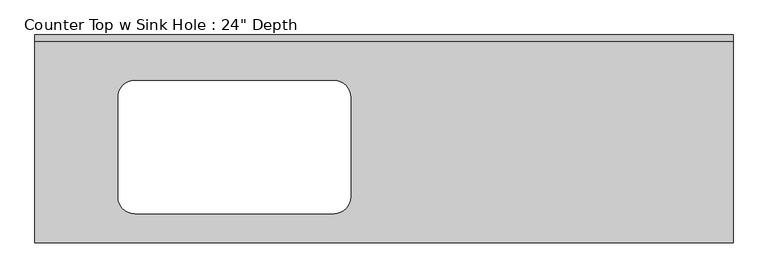
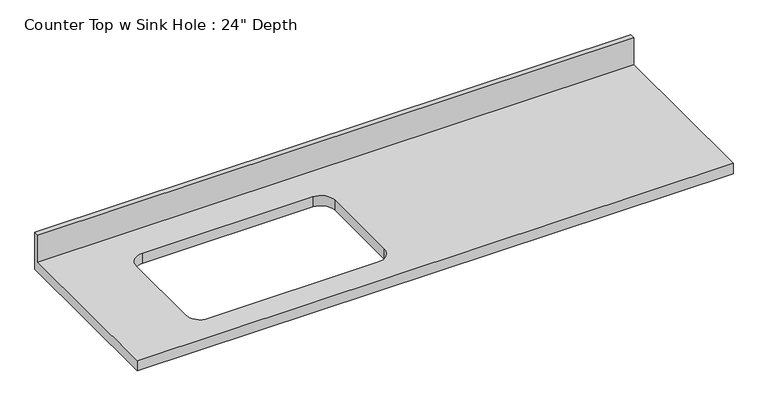
"""IFC4 building model written with IfcOpenShell, lengths in millimetres: furniture geometry."""

from ifc_helpers import new_model, si_unit, frame, origin, place, context, project, spatial, polyline, circle_curve, source, transform, mapped, element, save
from ifc_brep_helpers import plane_surface, revolved_surface, advanced_brep


def furniture_ac03d711(model_context):
    return source(origin(), model_context, "Body", "AdvancedBrep", [
        advanced_brep(
        [(-1200.4622951, -635.0, 914.4), (933.1377049, -635.0, 914.4), (933.1377049, -19.05, 914.4), (-1200.4622951, -19.05, 914.4), (-895.6622951, -139.7, 914.4), (-286.0622951, -139.7, 914.4), (-235.2622951, -190.5, 914.4), (-235.2622951, -495.3, 914.4), (-286.0622951, -546.1, 914.4), (-895.6622951, -546.1, 914.4), (-946.4622951, -495.3, 914.4), (-946.4622951, -190.5, 914.4), (933.1377049, 0.0, 876.3), (933.1377049, -635.0, 876.3), (-1200.4622951, -635.0, 876.3), (-1200.4622951, 0.0, 876.3), (-286.0622951, -139.7, 876.3), (-895.6622951, -139.7, 876.3), (-946.4622951, -190.5, 876.3), (-946.4622951, -495.3, 876.3), (-895.6622951, -546.1, 876.3), (-286.0622951, -546.1, 876.3), (-235.2622951, -495.3, 876.3), (-235.2622951, -190.5, 876.3), (-1200.4622951, 0.0, 1016.0), (933.1377049, 0.0, 1016.0), (-1200.4622951, -19.05, 1016.0), (933.1377049, -19.05, 1016.0)],
        [
            (0, 1),
            (1, 2),
            (2, 3),
            (3, 0),
            (4, 5),
            (5, 6, circle_curve(frame((-286.0622951, -190.5, 914.4), z_axis=(0.0, 0.0, -1.0), x_axis=(1.0, 0.0, 0.0)), 50.8)),
            (6, 7),
            (7, 8, circle_curve(frame((-286.0622951, -495.3, 914.4), z_axis=(0.0, 0.0, -1.0), x_axis=(1.0, 0.0, 0.0)), 50.8)),
            (8, 9),
            (9, 10, circle_curve(frame((-895.6622951, -495.3, 914.4), z_axis=(0.0, 0.0, -1.0), x_axis=(1.0, 0.0, 0.0)), 50.8)),
            (10, 11),
            (11, 4, circle_curve(frame((-895.6622951, -190.5, 914.4), z_axis=(0.0, 0.0, -1.0), x_axis=(1.0, 0.0, 0.0)), 50.8)),
            (12, 13),
            (13, 14),
            (14, 15),
            (15, 12),
            (16, 17),
            (17, 18, circle_curve(frame((-895.6622951, -190.5, 876.3), z_axis=(0.0, 0.0, 1.0), x_axis=(1.0, 0.0, 0.0)), 50.8)),
            (18, 19),
            (19, 20, circle_curve(frame((-895.6622951, -495.3, 876.3), z_axis=(0.0, 0.0, 1.0), x_axis=(1.0, 0.0, 0.0)), 50.8)),
            (20, 21),
            (21, 22, circle_curve(frame((-286.0622951, -495.3, 876.3), z_axis=(0.0, 0.0, 1.0), x_axis=(1.0, 0.0, 0.0)), 50.8)),
            (22, 23),
            (23, 16, circle_curve(frame((-286.0622951, -190.5, 876.3), z_axis=(0.0, 0.0, 1.0), x_axis=(1.0, 0.0, 0.0)), 50.8)),
            (15, 24),
            (24, 25),
            (25, 12),
            (14, 0),
            (3, 26),
            (26, 24),
            (13, 1),
            (25, 27),
            (27, 2),
            (4, 17),
            (16, 5),
            (11, 18),
            (10, 19),
            (9, 20),
            (8, 21),
            (7, 22),
            (6, 23),
            (26, 27),
        ],
        [
            plane_surface(frame((-1200.4622951, 0.0, 914.4), z_axis=(0.0, 0.0, 1.0), x_axis=(-1.0, 0.0, 0.0))),
            plane_surface(frame((-1200.4622951, 0.0, 876.3), z_axis=(0.0, 0.0, -1.0), x_axis=(1.0, 0.0, 0.0))),
            plane_surface(frame((933.1377049, 0.0, 914.4), z_axis=(0.0, 1.0, 0.0), x_axis=(0.0, 0.0, -1.0))),
            plane_surface(frame((-1200.4622951, 0.0, 914.4), z_axis=(-1.0, 0.0, 0.0), x_axis=(0.0, 0.0, -1.0))),
            plane_surface(frame((-1200.4622951, -635.0, 914.4), z_axis=(0.0, -1.0, 0.0), x_axis=(0.0, 0.0, -1.0))),
            plane_surface(frame((933.1377049, -635.0, 914.4), z_axis=(1.0, 0.0, 0.0), x_axis=(0.0, 0.0, -1.0))),
            plane_surface(frame((-286.0622951, -139.7, 914.4), z_axis=(0.0, -1.0, 0.0), x_axis=(0.0, 0.0, -1.0))),
            revolved_surface(polyline([(-844.8622951000001, -190.5, 914.4), (-844.8622951000001, -190.5, 876.3)]), (-895.6622951, -190.5, 876.3), (0.0, 0.0, 1.0)),
            plane_surface(frame((-946.4622951, -190.5, 914.4), z_axis=(1.0, 0.0, 0.0), x_axis=(0.0, 0.0, -1.0))),
            revolved_surface(polyline([(-844.8622951000001, -495.3, 914.4), (-844.8622951000001, -495.3, 876.3)]), (-895.6622951, -495.3, 876.3), (0.0, 0.0, 1.0)),
            plane_surface(frame((-895.6622951, -546.1, 914.4), z_axis=(0.0, 1.0, 0.0), x_axis=(0.0, 0.0, -1.0))),
            revolved_surface(polyline([(-235.26229509999996, -495.3, 914.4), (-235.26229509999996, -495.3, 876.3)]), (-286.0622951, -495.3, 876.3), (0.0, 0.0, 1.0)),
            plane_surface(frame((-235.2622951, -495.3, 914.4), z_axis=(-1.0, 0.0, 0.0), x_axis=(0.0, 0.0, -1.0))),
            revolved_surface(polyline([(-235.26229509999996, -190.5, 914.4), (-235.26229509999996, -190.5, 876.3)]), (-286.0622951, -190.5, 876.3), (0.0, 0.0, 1.0)),
            plane_surface(frame((-1200.4622951, 0.0, 1016.0), z_axis=(0.0, 0.0, 1.0), x_axis=(0.0, -1.0, 0.0))),
            plane_surface(frame((-1200.4622951, -19.05, 1016.0), z_axis=(0.0, -1.0, 0.0), x_axis=(0.0, 0.0, -1.0))),
        ],
        [
            (0, [[1, 2, 3, 4], [5, 6, 7, 8, 9, 10, 11, 12]]),
            (1, [[13, 14, 15, 16], [17, 18, 19, 20, 21, 22, 23, 24]]),
            (2, [[-16, 25, 26, 27]]),
            (3, [[-15, 28, -4, 29, 30, -25]]),
            (4, [[-1, -28, -14, 31]]),
            (5, [[-13, -27, 32, 33, -2, -31]]),
            (6, [[34, -17, 35, -5]]),
            (7, [[-34, -12, 36, -18]]),
            (8, [[-36, -11, 37, -19]]),
            (9, [[-37, -10, 38, -20]]),
            (10, [[-38, -9, 39, -21]]),
            (11, [[-39, -8, 40, -22]]),
            (12, [[-40, -7, 41, -23]]),
            (13, [[-35, -24, -41, -6]]),
            (14, [[-30, 42, -32, -26]]),
            (15, [[-42, -29, -3, -33]]),
        ],
    ),
    ])


if __name__ == "__main__":
    model = new_model("IFC4")
    model_context = context("Model", 3, world=origin())
    ifc_project = project(units=[si_unit("LENGTHUNIT", "METRE", prefix="MILLI")], contexts=[model_context])
    site = spatial("IfcSite", under=ifc_project)
    building = spatial("IfcBuilding", under=site)
    placement = place(None, origin())
    furniture_shape = furniture_ac03d711(model_context)
    element("IfcFurniture", 1, ObjectType="Counter Top w Sink Hole : 24\" Depth", at=placement, inside=building, context=model_context, shape_type="MappedRepresentation", body=[
        mapped(furniture_shape, transform((0.0, 0.0, 0.0), x_axis=(1.0, 0.0, 0.0), y_axis=(0.0, 1.0, 0.0), z_axis=(0.0, 0.0, 1.0))),
    ])
    save(model, "model.ifc")

# Revit data of these elements
# Type "Counter Top w Sink Hole : 24\" Depth"
#   Assembly Code = "C1030400"
#   Counter Thickness = 0' - 1 1/2"
#   Depth = 2' - 1"
#   Height = 3' - 0"
#   Length [instance default] = 8' - 0"
#   Sink Location [instance default] = 2' - 0"
#   Sink Location To Wall [instance default] = 0' - 6"
#   Sink Opening Depth [instance default] = 1' - 3"
#   Sink Opening Width [instance default] = 2' - 3"
#   Counter Top Material = none
#   Default Elevation = 0
# Element 1 (IfcFurniture, "Counter Top w Sink Hole : 24\" Depth")
#   Length = 7' - 0"
#   Materials on its faces: "Counter Top"
# Materials
#   "Counter Top": class "Wood", colour RGB 226 177 128, transparency 0
